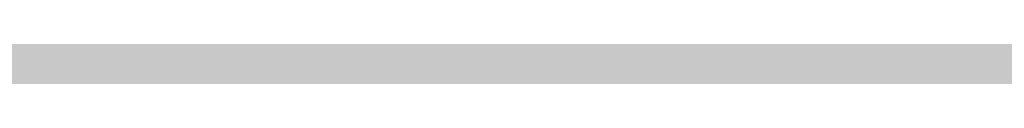
# Model space of a CAD drawing. Units: feet. Extents: x 3168 to 4724, y 827 to 1477.
# Tile 80 of 256: x 3273.6101 to 3274.1481, y 1099.0007 to 1099.0148. Entities that reach past the tile are written whole.
import ezdxf

# ---------------------------------------------------------------- set-up
doc = ezdxf.new("R2010")
doc.units = ezdxf.units.FT
doc.layers.add('A-ELEV', color=7, linetype='Continuous', lineweight=35)
doc.layers.add('A-ELEV-PATT', color=8, linetype='Continuous', lineweight=13)

msp = doc.modelspace()

# ---------------------------------------------------------------- hatches: boundary and pattern name
at = {"layer": 'A-ELEV-PATT'}
h = msp.add_hatch(color=256, dxfattribs=at)
h.dxf.hatch_style = 1
edge = h.paths.add_edge_path()
edge.add_ellipse((3552.90576, 979.22014), major_axis=(36.74492, 0), ratio=0.48484848, start_angle=0, end_angle=360)
edge = h.paths.add_edge_path()
edge.add_ellipse((3559.89164, 929.25228), major_axis=(36.74492, 0), ratio=0.48484848, start_angle=0, end_angle=360)
edge = h.paths.add_edge_path()
edge.add_line((3299.31681, 1198.60608), (3479.91671, 1198.60608))
edge.add_line((3479.91671, 1198.60608), (3479.91671, 1209.86857))
edge.add_spline(control_points=[(3479.91671, 1209.86857), (3464.30116, 1209.86857), (3448.6856, 1209.86857), (3410.94914, 1209.86857), (3388.82823, 1209.86857), (3355.64688, 1209.86857), (3344.58642, 1209.86857), (3327.99574, 1209.86857), (3322.46552, 1209.86857), (3314.17018, 1209.86857), (3311.40507, 1209.86857), (3307.2574, 1209.86857), (3305.87484, 1209.86857), (3303.801, 1209.86857), (3303.10973, 1209.86857), (3302.07281, 1209.86857), (3301.72717, 1209.86857), (3301.20871, 1209.86857), (3301.03589, 1209.86857), (3300.77666, 1209.86857), (3300.69025, 1209.86857), (3300.56064, 1209.86857), (3300.51743, 1209.86857), (3300.45263, 1209.86857), (3300.43102, 1209.86857), (3300.39862, 1209.86857), (3300.38782, 1209.86857), (3300.36622, 1209.86857), (3300.34568, 1209.86857), (3300.34555, 1209.86857), (3300.3455, 1209.86857), (3300.3433, 1209.86857), (3300.34115, 1209.86857), (3300.33791, 1209.86857), (3300.33683, 1209.86857), (3300.33394, 1209.86857), (3300.33213, 1209.86857), (3300.32552, 1209.86858), (3300.32071, 1209.86858), (3300.31092, 1209.86859), (3300.30595, 1209.8686), (3300.29051, 1209.86862), (3300.28005, 1209.86865), (3300.23243, 1209.86878), (3300.1953, 1209.86895), (3299.95107, 1209.87061), (3299.74482, 1209.87433), (3299.43683, 1209.88326), (3299.33439, 1209.88679), (3299.18108, 1209.89292), (3299.13003, 1209.8951), (3298.65222, 1209.9168), (3298.22946, 1209.94572), (3297.60163, 1210.00237), (3297.3934, 1210.02346), (3297.08265, 1210.05831), (3296.97933, 1210.07046), (3296.29295, 1210.15486), (3295.71815, 1210.24336), (3294.86872, 1210.39885), (3294.5877, 1210.45448), (3294.16934, 1210.54335), (3294.03042, 1210.57388), (3291.70715, 1211.1012), (3289.65359, 1211.81344), (3285.77626, 1213.56399), (3283.95141, 1214.60348), (3280.51216, 1216.98008), (3278.89724, 1218.31759), (3276.37991, 1220.82949), (3275.41604, 1221.91774), (3274.03934, 1223.7077), (3273.58104, 1224.34953), (3273.14323, 1225.01632)], knot_values=[39.119033, 39.119033, 39.119033, 39.119033, 39.286353, 39.286353, 39.523379, 39.523379, 39.641892, 39.641892, 39.701148, 39.701148, 39.730777, 39.730777, 39.745591, 39.745591, 39.752998, 39.752998, 39.756701, 39.756701, 39.758553, 39.758553, 39.759479, 39.759479, 39.759942, 39.759942, 39.760173, 39.760173, 39.760289, 39.760289, 39.760405, 39.760405, 39.760463, 39.760463, 39.763389, 39.763389, 39.764851, 39.764851, 39.767304, 39.767304, 39.773825, 39.773825, 39.78057, 39.78057, 39.79477, 39.79477, 39.845194, 39.845194, 40.126715, 40.126715, 40.267476, 40.267476, 40.337856, 40.337856, 40.927023, 40.927023, 41.221606, 41.221606, 41.368898, 41.368898, 42.202622, 42.202622, 42.619485, 42.619485, 42.827916, 42.827916, 46.118323, 46.118323, 49.408731, 49.408731, 52.699139, 52.699139, 54.927489, 54.927489, 56.104228, 56.104228, 56.104228, 56.104228], weights=[1, 1, 1, 1, 1, 1, 1, 1, 1, 1, 1, 1, 1, 1, 1, 1, 1, 1, 1, 1, 1, 1, 1, 1, 1, 1, 1, 1, 1, 1, 1, 1, 1, 1, 1, 1, 1, 1, 1, 1, 1, 1, 1, 1, 1, 1, 1, 1, 1, 1, 1, 1, 1, 1, 1, 1, 1, 1, 1, 1, 1, 1, 1, 1, 1, 1, 1, 1, 1, 1, 1, 1, 1, 1], degree=3, periodic=0)
edge.add_line((3273.14323, 1225.01632), (3273.14323, 1099.01632))
edge.add_line((3273.14323, 1099.01632), (3299.31681, 1099.01632))
edge.add_line((3299.31681, 1099.01632), (3299.31681, 1198.60608))
edge = h.paths.add_edge_path()
edge.add_line((3304.75844, 1324.15806), (3479.91671, 1324.15806))
edge.add_line((3479.91671, 1324.15806), (3479.91671, 1335.71462))
edge.add_line((3479.91671, 1335.71462), (3269.16163, 1335.71462))
edge.add_spline(control_points=[(3269.16163, 1335.71462), (3264.02423, 1335.71462), (3258.36412, 1328.95819), (3259.26431, 1323.90027)], knot_values=[0, 0, 0, 0, 15.412191, 15.412191, 15.412191, 15.412191], degree=3, periodic=0)
edge.add_line((3259.26431, 1323.90027), (3265.51685, 1288.76913))
edge.add_line((3265.51685, 1288.76913), (3275.2651, 1261.54563))
edge.add_line((3275.2651, 1261.54563), (3304.75844, 1261.54563))
edge.add_line((3304.75844, 1261.54563), (3304.75844, 1324.15806))
h = msp.add_hatch(color=256, dxfattribs=at)
h.dxf.hatch_style = 1
h.paths.add_polyline_path([(3384.52525, 1099.01632), (3335.02917, 1099.01632), (3299.31681, 1099.01632), (3273.14323, 1099.01632), (3217.56536, 1099.01632), (3168.06928, 827.11626), (3335.02917, 827.11626)])

# ---------------------------------------------------------------- linework, layer by layer
at = {"layer": 'A-ELEV'}
msp.add_open_spline([(3808.5202, 1099.01632), (3808.5202, 1141.41324), (3808.5202, 1183.81015), (3808.5202, 1226.63532), (3808.5202, 1227.06358), (3808.5202, 1227.49183), (3811.49187, 1248.99467), (3814.46354, 1270.49752), (3817.46523, 1292.21756), (3817.49525, 1292.43476), (3817.52526, 1292.65196), (3817.5728, 1310.10675), (3817.62034, 1327.56153), (3817.66788, 1345.01632), (3817.66788, 1345.45796), (3817.66788, 1345.89961), (3817.66788, 1346.45605), (3817.66788, 1346.57084), (3817.66788, 1346.75289), (3817.66788, 1346.82014), (3817.66788, 1346.93487), (3817.66788, 1346.98234), (3817.66788, 1347.03859), (3817.66788, 1347.04736), (3817.66788, 1347.07366), (3817.66788, 1347.0593), (3817.66788, 1347.06155), (3817.66788, 1347.06267), (3817.66788, 1347.06603), (3817.66787, 1347.06827), (3817.66787, 1347.075), (3817.66787, 1347.07949), (3817.66785, 1347.09294), (3817.66783, 1347.1019), (3817.66777, 1347.12879), (3817.6677, 1347.1467), (3817.66743, 1347.20042), (3817.66716, 1347.23619), (3817.6661, 1347.34338), (3817.66504, 1347.41469), (3817.66081, 1347.62809), (3817.65661, 1347.76971), (3817.63997, 1348.19249), (3817.62351, 1348.47159), (3817.55909, 1349.30007), (3817.49612, 1349.84059), (3817.25543, 1351.42416), (3817.02632, 1352.42879), (3816.30687, 1354.88891), (3815.74375, 1356.26873), (3814.46396, 1358.81921), (3813.74641, 1359.99097), (3812.19584, 1362.17234), (3811.36225, 1363.18212), (3809.58884, 1365.06901), (3808.64882, 1365.94611), (3806.65426, 1367.57962), (3805.5997, 1368.33615), (3803.35289, 1369.72233), (3802.16054, 1370.35239), (3799.60081, 1371.45359), (3798.23269, 1371.92548), (3795.28008, 1372.63462), (3793.69315, 1372.87207), (3791.86944, 1372.92648), (3791.74086, 1372.92922), (3791.35337, 1372.9341), (3791.09271, 1372.9329), (3790.30412, 1372.91507), (3789.76954, 1372.88419), (3789.20919, 1372.83024), (3789.19062, 1372.82842), (3789.13489, 1372.82291), (3789.0977, 1372.81914), (3789.04844, 1372.81401), (3789.0364, 1372.81274), (3789.00026, 1372.80892), (3788.97615, 1372.80633), (3788.9494, 1372.8034), (3788.94679, 1372.80312), (3788.94257, 1372.80266), (3788.94097, 1372.80248), (3788.93857, 1372.80222), (3788.93778, 1372.80213), (3788.93539, 1372.80187), (3788.86753, 1372.7944), (3788.75687, 1372.78223), (3788.70153, 1372.77614), (3788.53553, 1372.75788), (3788.42486, 1372.74571), (3788.09286, 1372.70918), (3787.87152, 1372.68484), (3787.20751, 1372.61179), (3786.76483, 1372.5631), (3785.43681, 1372.41701), (3784.55147, 1372.31962), (3781.89542, 1372.02744), (3780.12473, 1371.83266), (3774.81265, 1371.24831), (3771.27126, 1370.85874), (3760.64709, 1369.69004), (3753.56431, 1368.9109), (3732.31597, 1366.5735), (3718.15042, 1365.01523), (3694.00676, 1362.35933), (3684.02866, 1361.26169), (3674.05056, 1360.16406), (3664.60066, 1360.16406), (3655.15077, 1360.16406), (3626.80108, 1360.16406), (3607.90129, 1360.16406), (3551.20192, 1360.16406), (3513.40234, 1360.16406), (3467.72518, 1360.16406), (3459.8476, 1360.16406), (3436.21487, 1360.16406), (3420.45972, 1360.16406), (3373.19425, 1360.16406), (3341.68395, 1360.16406), (3302.84816, 1360.16406), (3295.52269, 1360.16406), (3286.03829, 1360.16406), (3283.87937, 1360.16406), (3277.40261, 1360.16406), (3273.08477, 1360.16406), (3267.73285, 1360.16406), (3266.69877, 1360.16406), (3263.59652, 1360.16406), (3261.52835, 1360.16406), (3259.23694, 1360.16406), (3259.0137, 1360.16406), (3258.34396, 1360.16406), (3257.89747, 1360.16406), (3257.431, 1360.16406), (3257.41102, 1360.16406), (3257.37057, 1360.16406), (3257.37547, 1360.16406), (3257.3746, 1360.16406), (3257.37394, 1360.16406), (3257.37196, 1360.16406), (3257.37064, 1360.16406), (3257.36667, 1360.16406), (3257.36403, 1360.16406), (3257.35611, 1360.16405), (3257.35083, 1360.16405), (3257.33499, 1360.16402), (3257.32443, 1360.164), (3257.29277, 1360.1639), (3257.27168, 1360.1638), (3257.20844, 1360.1634), (3257.16634, 1360.163), (3257.04021, 1360.16139), (3256.95635, 1360.15978), (3256.7055, 1360.15339), (3256.53924, 1360.14704), (3256.04357, 1360.12192), (3255.7173, 1360.0971), (3254.75245, 1360.00048), (3254.12797, 1359.90651), (3252.18007, 1359.52533), (3250.94157, 1359.14399), (3248.67018, 1358.24329), (3247.63574, 1357.72383), (3245.73263, 1356.60347), (3244.86339, 1356.00206), (3243.25311, 1354.74287), (3242.51197, 1354.08473), (3240.75105, 1352.34478), (3239.80096, 1351.22957), (3238.08777, 1348.87244), (3237.32469, 1347.63036), (3235.98251, 1344.97163), (3235.40221, 1343.55491), (3234.59108, 1340.81546), (3234.31088, 1339.54355), (3233.97649, 1336.80256), (3233.92211, 1335.33088), (3234.14892, 1332.59127), (3234.34953, 1331.3672), (3234.71989, 1329.99937), (3234.75242, 1329.88336), (3234.85362, 1329.5348), (3234.92589, 1329.30168), (3235.02484, 1329.00255), (3235.04692, 1328.93693), (3235.07764, 1328.84724), (3235.08592, 1328.8232), (3235.11094, 1328.75106), (3235.12783, 1328.70296), (3235.14799, 1328.64624), (3235.15106, 1328.63763), (3235.1561, 1328.62353), (3235.15806, 1328.61803), (3235.16021, 1328.61203), (3235.16561, 1328.59694), (3235.1801, 1328.55649), (3235.19026, 1328.5281), (3235.22076, 1328.44295), (3235.24108, 1328.38618), (3235.30207, 1328.21587), (3235.34273, 1328.10232), (3235.4647, 1327.7617), (3235.54601, 1327.53462), (3235.78995, 1326.85338), (3235.95258, 1326.39922), (3236.44046, 1325.03674), (3236.76571, 1324.12841), (3237.74148, 1321.40345), (3238.39198, 1319.5868), (3240.34351, 1314.13687), (3241.64452, 1310.50358), (3245.54757, 1299.60371), (3248.14961, 1292.33713), (3255.95571, 1270.53739), (3261.15977, 1256.00423), (3267.38762, 1238.612), (3268.4114, 1235.75294), (3269.51038, 1232.68386), (3269.58558, 1232.47385), (3269.70661, 1232.13585), (3269.75244, 1232.00786), (3269.82733, 1231.79873), (3269.85638, 1231.7176), (3269.90632, 1231.57812), (3269.92721, 1231.51978), (3269.97247, 1231.39341), (3269.99683, 1231.32537), (3270.0265, 1231.24251), (3270.03181, 1231.22768), (3270.04028, 1231.20402), (3270.03922, 1231.20698), (3270.03936, 1231.2066), (3270.03943, 1231.20641), (3270.03963, 1231.20585), (3270.03977, 1231.20547), (3270.04017, 1231.20433), (3270.04044, 1231.20358), (3270.04125, 1231.20131), (3270.0418, 1231.1998), (3270.04342, 1231.19527), (3270.0445, 1231.19225), (3270.04776, 1231.18318), (3270.04993, 1231.17714), (3270.05644, 1231.15903), (3270.06079, 1231.14696), (3270.07387, 1231.11076), (3270.08261, 1231.08666), (3270.10894, 1231.01441), (3270.1266, 1230.96635), (3270.17993, 1230.82246), (3270.21595, 1230.72692), (3270.32532, 1230.44151), (3270.40003, 1230.25281), (3270.62925, 1229.69144), (3270.78888, 1229.3235), (3271.28649, 1228.23832), (3271.6431, 1227.53975), (3272.77586, 1225.51528), (3273.61417, 1224.2605), (3275.41604, 1221.91774), (3276.37991, 1220.82949), (3278.89724, 1218.31759), (3280.51216, 1216.98008), (3283.95141, 1214.60348), (3285.77626, 1213.56399), (3289.65359, 1211.81344), (3291.70715, 1211.1012), (3294.03042, 1210.57388), (3294.16934, 1210.54335), (3294.5877, 1210.45448), (3294.86872, 1210.39885), (3295.71815, 1210.24336), (3296.29295, 1210.15486), (3296.97933, 1210.07046), (3297.08265, 1210.05831), (3297.3934, 1210.02346), (3297.60163, 1210.00237), (3298.22946, 1209.94572), (3298.65222, 1209.9168), (3299.13003, 1209.8951), (3299.18108, 1209.89292), (3299.33439, 1209.88679), (3299.43683, 1209.88326), (3299.74482, 1209.87433), (3299.95107, 1209.87061), (3300.1953, 1209.86895), (3300.23243, 1209.86878), (3300.28005, 1209.86865), (3300.29051, 1209.86862), (3300.30595, 1209.8686), (3300.31092, 1209.86859), (3300.32071, 1209.86858), (3300.32552, 1209.86858), (3300.33213, 1209.86857), (3300.33394, 1209.86857), (3300.33683, 1209.86857), (3300.33791, 1209.86857), (3300.34115, 1209.86857), (3300.3433, 1209.86857), (3300.3455, 1209.86857), (3300.34555, 1209.86857), (3300.34568, 1209.86857), (3300.36622, 1209.86857), (3300.38782, 1209.86857), (3300.39862, 1209.86857), (3300.43102, 1209.86857), (3300.45263, 1209.86857), (3300.51743, 1209.86857), (3300.56064, 1209.86857), (3300.69025, 1209.86857), (3300.77666, 1209.86857), (3301.03589, 1209.86857), (3301.20871, 1209.86857), (3301.72717, 1209.86857), (3302.07281, 1209.86857), (3303.10973, 1209.86857), (3303.801, 1209.86857), (3305.87484, 1209.86857), (3307.2574, 1209.86857), (3311.40507, 1209.86857), (3314.17018, 1209.86857), (3322.46552, 1209.86857), (3327.99574, 1209.86857), (3344.58642, 1209.86857), (3355.64688, 1209.86857), (3388.82823, 1209.86857), (3410.94914, 1209.86857), (3477.31185, 1209.86857), (3521.55366, 1209.86857), (3566.83618, 1209.86857), (3567.87689, 1209.86857), (3570.99902, 1209.86857), (3573.08043, 1209.86857), (3575.7814, 1209.86857), (3576.40094, 1209.86857), (3577.29582, 1209.86857), (3577.57115, 1209.86857), (3578.39715, 1209.86857), (3578.94781, 1209.86857), (3579.75649, 1209.86857), (3580.01451, 1209.86857), (3580.34274, 1209.86857), (3580.32686, 1209.86857), (3580.32717, 1209.86857), (3580.32732, 1209.86857), (3580.32778, 1209.86857), (3580.32809, 1209.86857), (3580.329, 1209.86857), (3580.32961, 1209.86857), (3580.33145, 1209.86857), (3580.33267, 1209.86857), (3580.33633, 1209.86857), (3580.33878, 1209.86857), (3580.34611, 1209.86856), (3580.35099, 1209.86856), (3580.36566, 1209.86854), (3580.37544, 1209.86852), (3580.4048, 1209.86845), (3580.42439, 1209.86838), (3580.48318, 1209.86808), (3580.52244, 1209.86779), (3580.64036, 1209.86662), (3580.71919, 1209.86545), (3580.95632, 1209.86077), (3581.11522, 1209.85607), (3581.59416, 1209.83723), (3581.91642, 1209.81833), (3582.88995, 1209.74243), (3583.54799, 1209.66617), (3585.53183, 1209.36062), (3586.86722, 1209.05389), (3589.47155, 1208.25247), (3590.74024, 1207.75785), (3591.99545, 1207.1588), (3592.05781, 1207.12874), (3592.24424, 1207.03795), (3592.36768, 1206.97663), (3592.73528, 1206.79036), (3592.97675, 1206.6631), (3593.24454, 1206.51644), (3593.27473, 1206.49982), (3593.36512, 1206.44984), (3593.42511, 1206.41633), (3593.60431, 1206.31529), (3593.72273, 1206.24721), (3593.85721, 1206.1684), (3593.87436, 1206.15832), (3593.92574, 1206.12804), (3593.9599, 1206.1078), (3594.06209, 1206.0469), (3594.12983, 1206.00607), (3594.20844, 1205.95817), (3594.21968, 1205.9513), (3594.25339, 1205.93069), (3594.27582, 1205.91692), (3594.34297, 1205.87554), (3594.38756, 1205.84785), (3594.43362, 1205.81905), (3594.43526, 1205.81802), (3594.44017, 1205.81495), (3594.44345, 1205.81289), (3594.44712, 1205.81059), (3594.44752, 1205.81035), (3594.44869, 1205.80961), (3594.44948, 1205.80912), (3594.45037, 1205.80856), (3594.45047, 1205.8085), (3594.4506, 1205.80842), (3594.4674, 1205.79789), (3594.49327, 1205.78167), (3594.5062, 1205.77357), (3594.54501, 1205.74925), (3594.57088, 1205.73303), (3594.64849, 1205.6844), (3594.70023, 1205.65197), (3594.85544, 1205.55469), (3594.95892, 1205.48984), (3595.26936, 1205.29528), (3595.47631, 1205.16558), (3596.09719, 1204.77646), (3596.5111, 1204.51705), (3597.75284, 1203.73883), (3598.58067, 1203.22001), (3601.06415, 1201.66355), (3602.71981, 1200.62591), (3607.68677, 1197.513), (3610.99809, 1195.43773), (3620.93202, 1189.2119), (3627.55464, 1185.06135), (3647.42251, 1172.60971), (3660.66775, 1164.30861), (3700.40348, 1139.40531), (3726.89397, 1122.80312), (3757.20572, 1103.80605), (3761.02697, 1101.41118), (3764.84822, 1099.01632), (3745.32827, 1099.01632), (3725.80832, 1099.01632), (3706.28837, 1099.01632), (3706.28837, 1108.45324), (3706.28837, 1117.89016), (3706.28837, 1127.32708), (3710.75075, 1127.32708), (3715.21314, 1127.32708), (3719.67553, 1127.32708)], degree=3, knots=[0, 0, 0, 0, 0.982037, 0.982037, 0.991957, 0.991957, 0.991957, 1.966522, 1.966522, 1.976367, 1.976367, 1.976367, 2.976367, 2.976367, 2.976367, 3.00169, 3.00169, 3.008272, 3.008272, 3.012129, 3.012129, 3.014851, 3.014851, 3.015353, 3.015353, 3.016359, 3.016359, 3.017365, 3.017365, 3.019376, 3.019376, 3.023398, 3.023398, 3.031442, 3.031442, 3.047531, 3.047531, 3.079708, 3.079708, 3.144063, 3.144063, 3.272772, 3.272772, 3.53019, 3.53019, 4.045026, 4.045026, 5.074698, 5.074698, 6.700878, 6.700878, 8.327058, 8.327058, 9.953238, 9.953238, 11.579418, 11.579418, 13.205598, 13.205598, 14.831778, 14.831778, 16.457958, 16.457958, 18.084138, 18.084138, 18.206872, 18.206872, 18.45234, 18.45234, 18.943275, 18.943275, 18.960093, 18.960093, 18.993729, 18.993729, 19.00461, 19.00461, 19.026374, 19.026374, 19.028737, 19.028737, 19.03018, 19.03018, 19.030897, 19.030897, 19.032332, 19.032332, 19.033766, 19.033766, 19.036636, 19.036636, 19.042374, 19.042374, 19.053851, 19.053851, 19.076805, 19.076805, 19.122714, 19.122714, 19.21453, 19.21453, 19.398163, 19.398163, 19.765429, 19.765429, 20.024128, 20.024128, 20.024128, 20.092031, 20.092031, 20.227836, 20.227836, 20.499446, 20.499446, 20.556051, 20.556051, 20.66926, 20.66926, 20.895678, 20.895678, 20.948316, 20.948316, 20.963829, 20.963829, 20.994855, 20.994855, 21.002285, 21.002285, 21.017146, 21.017146, 21.01875, 21.01875, 21.021959, 21.021959, 21.022102, 21.022102, 21.022249, 21.022249, 21.022708, 21.022708, 21.023627, 21.023627, 21.025464, 21.025464, 21.029138, 21.029138, 21.036486, 21.036486, 21.051183, 21.051183, 21.080575, 21.080575, 21.139361, 21.139361, 21.256932, 21.256932, 21.492073, 21.492073, 21.962356, 21.962356, 23.01002, 23.01002, 24.057684, 24.057684, 25.105348, 25.105348, 26.153011, 26.153011, 27.776787, 27.776787, 29.400562, 29.400562, 31.024337, 31.024337, 32.278801, 32.278801, 33.533265, 33.533265, 34.467568, 34.467568, 34.553971, 34.553971, 34.726776, 34.726776, 34.775309, 34.775309, 34.793079, 34.793079, 34.82862, 34.82862, 34.834979, 34.834979, 34.839039, 34.839039, 34.839411, 34.839411, 34.840285, 34.840285, 34.842034, 34.842034, 34.845531, 34.845531, 34.852525, 34.852525, 34.866512, 34.866512, 34.894488, 34.894488, 34.950439, 34.950439, 35.062342, 35.062342, 35.286147, 35.286147, 35.733758, 35.733758, 35.821815, 35.821815, 35.828283, 35.828283, 35.832225, 35.832225, 35.834724, 35.834724, 35.836521, 35.836521, 35.838617, 35.838617, 35.839073, 35.839073, 35.839345, 35.839345, 35.839617, 35.839617, 35.840161, 35.840161, 35.841249, 35.841249, 35.843425, 35.843425, 35.847778, 35.847778, 35.856482, 35.856482, 35.873891, 35.873891, 35.908709, 35.908709, 35.978345, 35.978345, 36.117617, 36.117617, 36.396161, 36.396161, 36.953248, 36.953248, 38.067423, 38.067423, 40.295772, 40.295772, 42.524122, 42.524122, 45.81453, 45.81453, 49.104937, 49.104937, 52.395345, 52.395345, 52.603776, 52.603776, 53.020639, 53.020639, 53.854363, 53.854363, 54.001655, 54.001655, 54.296238, 54.296238, 54.885405, 54.885405, 54.955785, 54.955785, 55.096546, 55.096546, 55.378067, 55.378067, 55.42849, 55.42849, 55.442691, 55.442691, 55.449436, 55.449436, 55.455957, 55.455957, 55.458409, 55.458409, 55.459872, 55.459872, 55.462798, 55.462798, 55.462856, 55.462856, 55.462972, 55.462972, 55.463088, 55.463088, 55.463319, 55.463319, 55.463782, 55.463782, 55.464708, 55.464708, 55.46656, 55.46656, 55.470263, 55.470263, 55.47767, 55.47767, 55.492484, 55.492484, 55.522112, 55.522112, 55.581369, 55.581369, 55.699882, 55.699882, 55.936907, 55.936907, 56.410959, 56.410959, 56.42211, 56.42211, 56.444413, 56.444413, 56.451051, 56.451051, 56.454001, 56.454001, 56.459901, 56.459901, 56.462666, 56.462666, 56.463418, 56.463418, 56.464171, 56.464171, 56.465675, 56.465675, 56.468684, 56.468684, 56.474702, 56.474702, 56.486738, 56.486738, 56.51081, 56.51081, 56.558955, 56.558955, 56.655243, 56.655243, 56.847821, 56.847821, 57.232975, 57.232975, 58.003284, 58.003284, 59.543901, 59.543901, 62.625137, 62.625137, 68.787607, 68.787607, 74.950078, 74.950078, 75.27336, 75.27336, 75.919923, 75.919923, 77.213051, 77.213051, 77.377769, 77.377769, 77.707206, 77.707206, 78.366079, 78.366079, 78.462532, 78.462532, 78.655436, 78.655436, 79.041245, 79.041245, 79.105735, 79.105735, 79.234714, 79.234714, 79.492672, 79.492672, 79.502197, 79.502197, 79.521249, 79.521249, 79.523534, 79.523534, 79.528103, 79.528103, 79.528682, 79.528682, 79.528885, 79.528885, 79.529089, 79.529089, 79.529495, 79.529495, 79.530308, 79.530308, 79.531935, 79.531935, 79.535187, 79.535187, 79.541693, 79.541693, 79.554704, 79.554704, 79.580725, 79.580725, 79.632769, 79.632769, 79.736856, 79.736856, 79.94503, 79.94503, 80.361377, 80.361377, 80.421435, 80.421435, 80.421435, 81.421435, 81.421435, 81.421435, 82.421435, 82.421435, 82.421435, 83.421435, 83.421435, 83.421435, 83.421435], dxfattribs=at)

doc.saveas('drawing.dxf')
